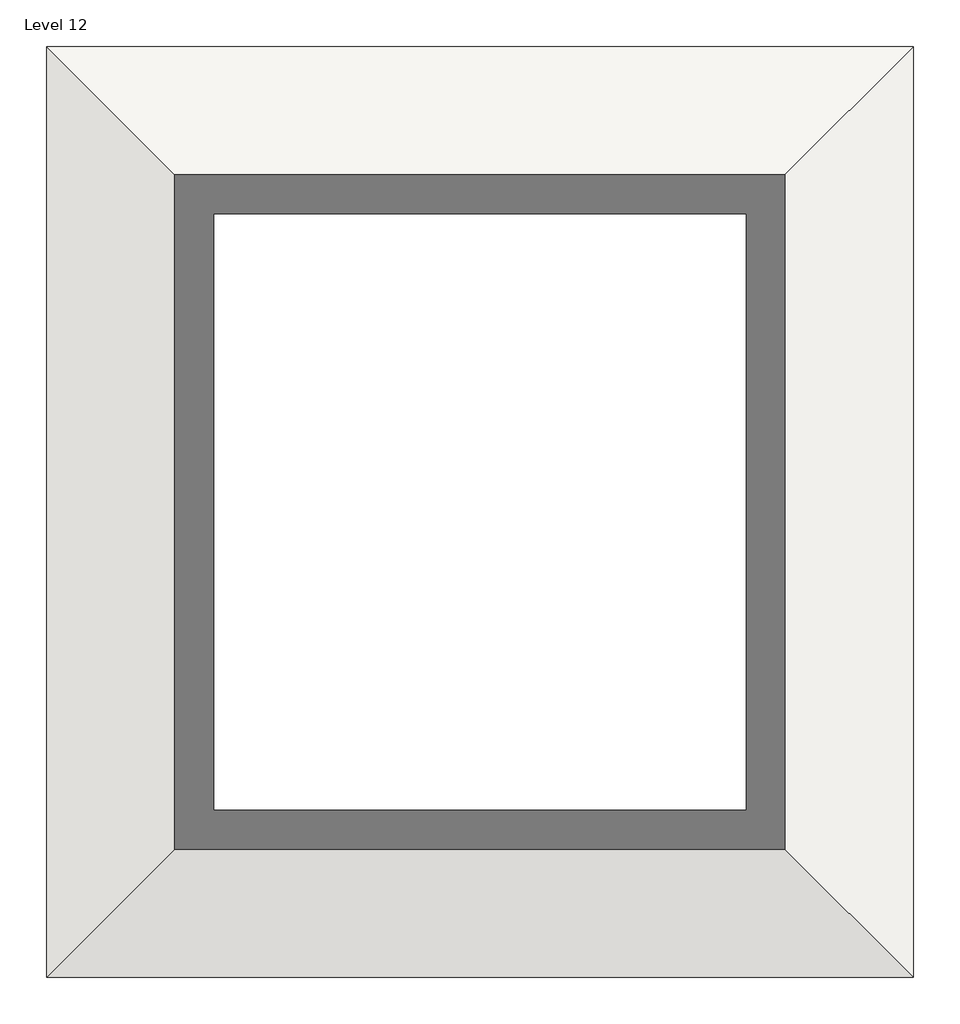
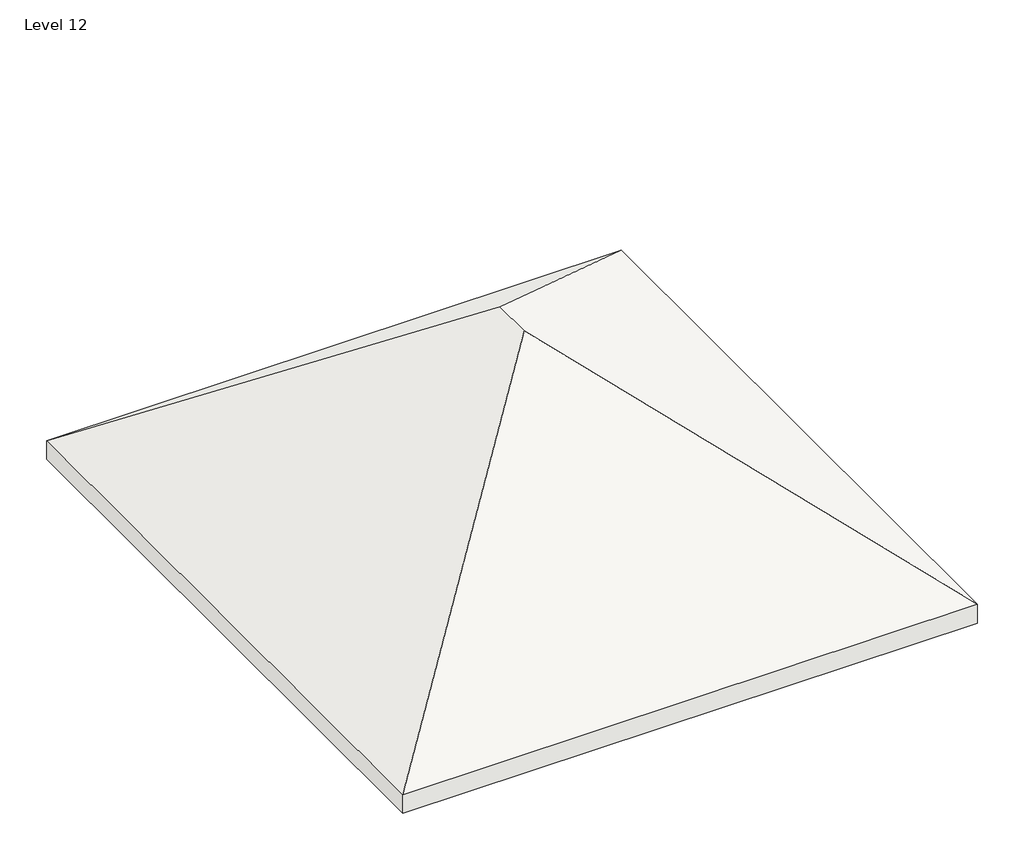
# One storey: 1 roof.
"""IFC4 building model written with IfcOpenShell, lengths in millimetres."""

from ifc_helpers import new_model, si_unit, origin, place, context, project, spatial, faceted_brep, element, save

model = new_model("IFC4")

# Units and contexts
model_context = context("Model", 3, world=origin())
ifc_project = project(units=[si_unit("LENGTHUNIT", "METRE", prefix="MILLI")], contexts=[model_context])

# Site, building, storey
site = spatial("IfcSite", under=ifc_project)
building = spatial("IfcBuilding", under=site)
storey = spatial("IfcBuildingStorey", under=building, Name="Level 12", Elevation=15925.8)

# Roof
placement = place(None, origin())
element("IfcRoof", 1, ObjectType="Generic - 9\"", at=placement, inside=storey, context=model_context, shape_type="Brep", body=[
    faceted_brep([(8102.4071875, 11141.9037429, 15925.8), (3962.2071875, 7001.7037429, 19030.95), (-177.9928125, 11141.9037429, 15925.8), (3962.2071875, 6392.1037429, 19030.95), (-177.9928125, 2251.9037429, 15925.8), (8102.4071875, 2251.9037429, 15925.8), (8102.4071875, 11141.9037429, 16211.55), (-177.9928125, 11141.9037429, 16211.55), (3962.2071875, 7001.7037429, 19316.7), (-177.9928125, 2251.9037429, 16211.55), (3962.2071875, 6392.1037429, 19316.7), (8102.4071875, 2251.9037429, 16211.55)], [[[0, 1, 2]], [[2, 1, 3, 4]], [[4, 3, 5]], [[1, 0, 5, 3]], [[6, 7, 8]], [[7, 9, 10, 8]], [[9, 11, 10]], [[6, 8, 10, 11]], [[2, 7, 6, 0]], [[4, 9, 7, 2]], [[5, 11, 9, 4]], [[0, 6, 11, 5]]]),
])

save(model, "model.ifc")

# Revit data of these elements
# Type "Generic - 9\""
#   Assembly Code = "B1020"
#   Layers, outside or top first: 0' - 9" no material (function 1)
# Element 1 (IfcRoof, "Generic - 9\"")
#   built-in parameter 1001705 = 63.375 (stored number, unit not read)
#   built-in parameter 1001710 = 33615
#   Phase Created = New Construction
#   Materials on its faces: "Default Roof"
# Materials
#   "Default Roof": colour RGB 88 101 114, transparency 0
